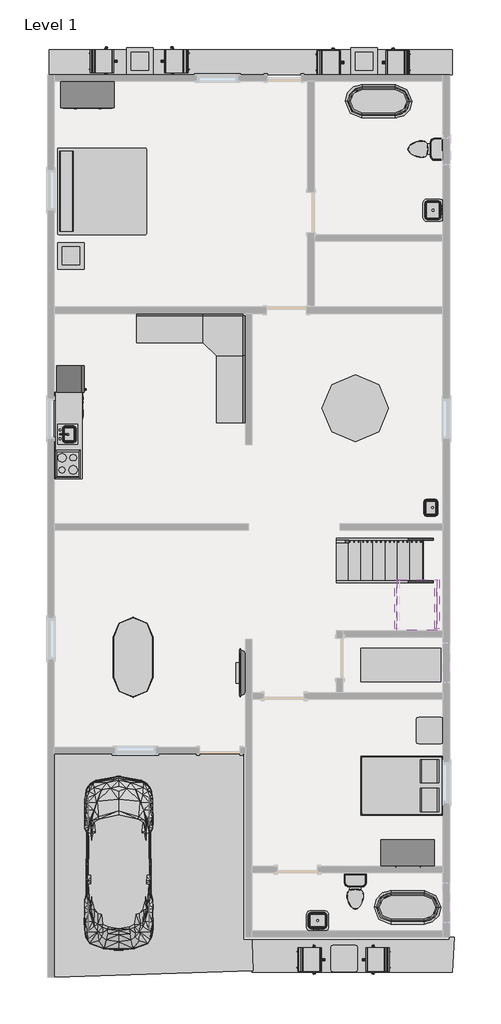
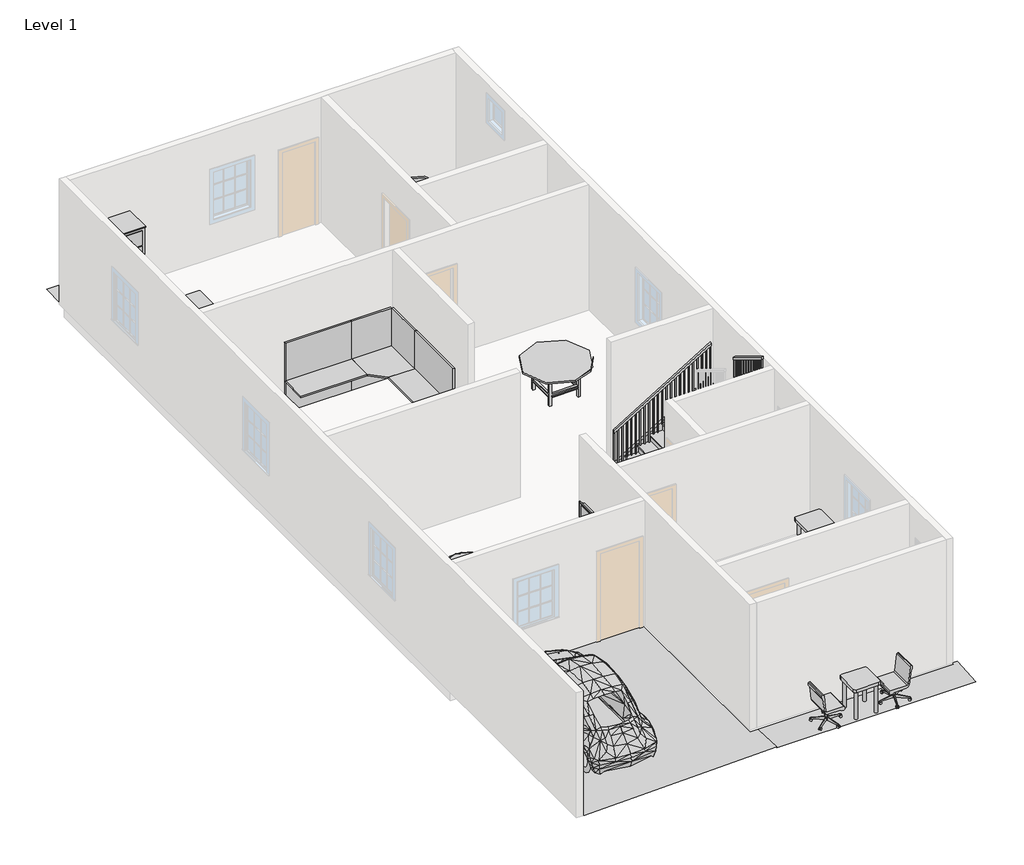
# One storey, part 2 of 2: 21 furniture elements, 8 flow terminals, 8 proxies, 4 members, 2 railings, 2 stair flights.
"""IFC4 building model written with IfcOpenShell, lengths in millimetres."""

from ifc_helpers import new_model, si_unit, frame, origin, place, context, project, spatial, polyline, outline, extrude, triangles, transform, mapped, element, save
from components import proxy_a6faaae8, proxy_45b28599, kitchenette_medium_kitchenette_medium_844211aa, rpc_beetle_rpc_beetle_3ce7ba48, proxy_c523a7b7, flow_terminal_871c2e40, flow_terminal_62a433f7, toilet_domestic_3d_toilet_domestic_3d_f7549cf7, toilet_domestic_3d_toilet_domestic_3d_183bbd19, flow_terminal_b374fae2, furniture_c8abb964, furniture_1fc5af50, chair_task_chair_task_b7f3823b, furniture_c6510c7c, furniture_9fa109b2, furniture_7a3aaa4f, furniture_b5c51a22, furniture_2c34a4f9, furniture_bbcc68ce, furniture_bcf351fa, furniture_a5b052b6, furniture_45e3acac, stair_flight_77e6af34, stair_flight_987ae6dc

model = new_model("IFC4")

# Units and contexts
model_context = context("Model", 3, world=origin())
ifc_project = project(units=[si_unit("LENGTHUNIT", "METRE", prefix="MILLI")], contexts=[model_context])

# Site, building, storey
site = spatial("IfcSite", under=ifc_project)
building = spatial("IfcBuilding", under=site)
storey = spatial("IfcBuildingStorey", under=building, Name="Level 1", Elevation=0.0)

# Proxies
placement = place(None, origin())
element("IfcBuildingElementProxy", 1, Name="Building Element Proxy", at=placement, inside=storey, context=model_context, shape_type="Tessellation", body=[
    triangles([(-7878.1871475, -7244.6450043, 0.0), (-7878.1871475, -8044.1648071, 0.0), (-3294.0675385, -8044.1648071, 0.0), (-3255.3873413, -7244.6450043, 0.0)], [[1, 2, 3], [3, 4, 1]], closed=False),
])
element("IfcBuildingElementProxy", 2, Name="Building Element Proxy", at=placement, inside=storey, context=model_context, shape_type="Tessellation", body=[
    triangles([(-12513.1071442, 13036.6751862, 0.0), (-12513.1071442, 12465.7553833, 0.0), (-3294.0675385, 13036.6751862, 0.0), (-3294.0675385, 12465.7553833, 0.0)], [[1, 2, 3], [4, 3, 2]], closed=False),
])
element("IfcBuildingElementProxy", 3, Name="Building Element Proxy", at=placement, inside=storey, context=model_context, shape_type="Tessellation", body=[
    triangles([(-12399.3873413, -3053.6450043, 0.0), (-8030.5871475, -3053.6450043, 0.0), (-7855.4362106, -8005.8386581, 0.0), (-12399.3873413, -8159.0450043, 0.0)], [[1, 4, 2], [3, 2, 4]], closed=False),
])
proxy_shape = proxy_a6faaae8(model_context)
element("IfcBuildingElementProxy", 4, Name="Cook Top-4 Unit2 : 22\" x 20\"", ObjectType="Cook Top-4 Unit2 : 22\" x 20\"", at=placement, inside=storey, context=model_context, shape_type="MappedRepresentation", body=[
    mapped(proxy_shape, transform((-12094.5873398, 3575.7549175, 0.0), x_axis=(0.0, 1.0000000000000002, 0.0), y_axis=(-1.0000000000000002, 0.0, 0.0), z_axis=(0.0, 0.0, 1.0))),
])
proxy_2_shape = proxy_45b28599(model_context)
element("IfcBuildingElementProxy", 5, Name="Dishwasher : 24\" x 24\" x 34\"", ObjectType="Dishwasher : 24\" x 24\" x 34\"", at=placement, inside=storey, context=model_context, shape_type="MappedRepresentation", body=[
    mapped(proxy_2_shape, transform((-11802.737775, 4526.937449, 0.0), x_axis=(0.0, 1.0000000000000002, 0.0), y_axis=(-1.0000000000000002, 0.0, 0.0), z_axis=(0.0, 0.0, 1.0))),
])
kitchenette_medium_kitchenette_medium_shape = kitchenette_medium_kitchenette_medium_844211aa(model_context)
element("IfcBuildingElementProxy", 6, Name="Kitchenette - Medium : Kitchenette - Medium", ObjectType="Kitchenette - Medium : Kitchenette - Medium", at=placement, inside=storey, context=model_context, shape_type="MappedRepresentation", body=[
    mapped(kitchenette_medium_kitchenette_medium_shape, transform((-12399.3873398, 3899.9172126, 0.0), x_axis=(0.0, 1.0000000000000002, 0.0), y_axis=(-1.0000000000000002, 0.0, 0.0), z_axis=(0.0, 0.0, 1.0))),
])
rpc_beetle_rpc_beetle_shape = rpc_beetle_rpc_beetle_3ce7ba48(model_context)
element("IfcBuildingElementProxy", 7, Name="RPC Beetle : RPC Beetle", ObjectType="RPC Beetle : RPC Beetle", at=placement, inside=storey, context=model_context, shape_type="MappedRepresentation", body=[
    mapped(rpc_beetle_rpc_beetle_shape, transform((-10926.1873398, -6787.4450825, 0.0), x_axis=(1.0, 0.0, 0.0), y_axis=(0.0, 1.0, 0.0), z_axis=(0.0, 0.0, 1.0))),
])
proxy_3_shape = proxy_c523a7b7(model_context)
element("IfcBuildingElementProxy", 8, Name="Refrigerator : 24\" x 25\" LH", ObjectType="Refrigerator : 24\" x 25\" LH", at=placement, inside=storey, context=model_context, shape_type="MappedRepresentation", body=[
    mapped(proxy_3_shape, transform((-12048.9383683, 5512.5049175, 0.0), x_axis=(0.0, 1.0000000000000002, 0.0), y_axis=(-1.0000000000000002, 0.0, 0.0), z_axis=(0.0, 0.0, 1.0))),
])

# Flow terminals
flow_terminal_shape = flow_terminal_871c2e40(model_context)
element("IfcFlowTerminal", 9, ObjectType="Sink Kitchen-Island : 18\" x 18\"", at=placement, inside=storey, context=model_context, shape_type="MappedRepresentation", body=[
    mapped(flow_terminal_shape, transform((-3753.0327409, 2588.1441581, 304.8), x_axis=(0.0, -1.0000000000000004, 0.0), y_axis=(1.0000000000000004, 0.0, 0.0), z_axis=(0.0, 0.0, 1.0))),
])
element("IfcFlowTerminal", 10, ObjectType="Sink Kitchen-Island : 18\" x 18\"", at=placement, inside=storey, context=model_context, shape_type="MappedRepresentation", body=[
    mapped(flow_terminal_shape, transform((-12092.2419387, 4233.165677, -14.4), x_axis=(0.0, 1.0000000000000002, 0.0), y_axis=(-1.0000000000000002, 0.0, 0.0), z_axis=(0.0, 0.0, 1.0))),
])
flow_terminal_2_shape = flow_terminal_62a433f7(model_context)
element("IfcFlowTerminal", 11, ObjectType="Sink Vanity-Square : 20\" x 18\"", at=placement, inside=storey, context=model_context, shape_type="MappedRepresentation", body=[
    mapped(flow_terminal_2_shape, transform((-6363.8980992, -6912.0996813, 304.8), x_axis=(-1.0, 0.0, 0.0), y_axis=(0.0, -1.0, 0.0), z_axis=(0.0, 0.0, 1.0))),
])
element("IfcFlowTerminal", 12, ObjectType="Sink Vanity-Square : 20\" x 18\"", at=placement, inside=storey, context=model_context, shape_type="MappedRepresentation", body=[
    mapped(flow_terminal_2_shape, transform((-3689.5327409, 9382.6441581, 304.8), x_axis=(0.0, -1.0000000000000002, 0.0), y_axis=(1.0000000000000002, 0.0, 0.0), z_axis=(0.0, 0.0, 1.0))),
])
toilet_domestic_3d_toilet_domestic_3d_shape = toilet_domestic_3d_toilet_domestic_3d_f7549cf7(model_context)
toilet_domestic_3d_toilet_domestic_3d_2_shape = toilet_domestic_3d_toilet_domestic_3d_183bbd19(model_context)
element("IfcFlowTerminal", 13, ObjectType="Toilet-Domestic-3D : Toilet-Domestic-3D", at=placement, inside=storey, context=model_context, shape_type="MappedRepresentation", body=[
    mapped(toilet_domestic_3d_toilet_domestic_3d_shape, transform((-5515.9873398, -6292.7490551, 0.0), x_axis=(1.0000000000000004, 0.0, 0.0), y_axis=(0.0, 1.0000000000000004, 0.0), z_axis=(0.0, 0.0, 1.0))),
    mapped(toilet_domestic_3d_toilet_domestic_3d_2_shape, transform((-5515.9873398, -6292.7490551, 0.0), x_axis=(1.0000000000000004, 0.0, 0.0), y_axis=(0.0, 1.0000000000000004, 0.0), z_axis=(0.0, 0.0, 1.0))),
])
element("IfcFlowTerminal", 14, ObjectType="Toilet-Domestic-3D : Toilet-Domestic-3D", at=placement, inside=storey, context=model_context, shape_type="MappedRepresentation", body=[
    mapped(toilet_domestic_3d_toilet_domestic_3d_shape, transform((-4004.0833671, 10763.9549175, 0.0), x_axis=(0.0, -1.0000000000000004, 0.0), y_axis=(1.0000000000000004, 0.0, 0.0), z_axis=(0.0, 0.0, 1.0))),
    mapped(toilet_domestic_3d_toilet_domestic_3d_2_shape, transform((-4004.0833671, 10763.9549175, 0.0), x_axis=(0.0, -1.0000000000000004, 0.0), y_axis=(1.0000000000000004, 0.0, 0.0), z_axis=(0.0, 0.0, 1.0))),
])
flow_terminal_3_shape = flow_terminal_b374fae2(model_context)
element("IfcFlowTerminal", 15, ObjectType="Tub-Free Standing-3D : 30\" x 60\"", at=placement, inside=storey, context=model_context, shape_type="MappedRepresentation", body=[
    mapped(flow_terminal_3_shape, transform((-4322.1873398, -6558.8450825, 0.0), x_axis=(0.0, -0.9999999999999998, 0.0), y_axis=(0.9999999999999998, 0.0, 0.0), z_axis=(0.0, 0.0, 1.0))),
])
element("IfcFlowTerminal", 16, ObjectType="Tub-Free Standing-3D : 30\" x 60\"", at=placement, inside=storey, context=model_context, shape_type="MappedRepresentation", body=[
    mapped(flow_terminal_3_shape, transform((-4982.5873398, 11856.1549175, 0.0), x_axis=(0.0, 1.0000000000000002, 0.0), y_axis=(-1.0000000000000002, 0.0, 0.0), z_axis=(0.0, 0.0, 1.0))),
])

# Furniture
furniture_shape = furniture_c8abb964(model_context)
element("IfcFurniture", 17, ObjectType="Bed-Box : Double 53\" x 74\"", at=placement, inside=storey, context=model_context, shape_type="MappedRepresentation", body=[
    mapped(furniture_shape, transform((-4214.7578316, -3438.3926234, 0.0), x_axis=(0.0, -1.0000000000000002, 0.0), y_axis=(1.0000000000000002, 0.0, 0.0), z_axis=(0.0, 0.0, 1.0))),
])
furniture_2_shape = furniture_1fc5af50(model_context)
element("IfcFurniture", 18, ObjectType="Bed-Standard : King 78\" x 80\"", at=placement, inside=storey, context=model_context, shape_type="MappedRepresentation", body=[
    mapped(furniture_2_shape, transform((-11352.7824218, 9527.266393, 0.0), x_axis=(0.0, 1.0000000000000002, 0.0), y_axis=(-1.0000000000000002, 0.0, 0.0), z_axis=(0.0, 0.0, 1.0))),
])
chair_task_chair_task_shape = chair_task_chair_task_b7f3823b(model_context)
element("IfcFurniture", 19, ObjectType="Chair-Task : Chair-Task", at=placement, inside=storey, context=model_context, shape_type="MappedRepresentation", body=[
    mapped(chair_task_chair_task_shape, transform((-4989.0414382, -7893.6359021, 0.0), x_axis=(0.0, 1.0000000000000009, 0.0), y_axis=(-1.0000000000000009, 0.0, 0.0), z_axis=(0.0, 0.0, 1.0))),
])
element("IfcFurniture", 20, ObjectType="Chair-Task : Chair-Task", at=placement, inside=storey, context=model_context, shape_type="MappedRepresentation", body=[
    mapped(chair_task_chair_task_shape, transform((-6576.3332414, -7611.6542628, 0.0), x_axis=(0.0, -1.0000000000000004, 0.0), y_axis=(1.0000000000000004, 0.0, 0.0), z_axis=(0.0, 0.0, 1.0))),
])
element("IfcFurniture", 21, ObjectType="Chair-Task : Chair-Task", at=placement, inside=storey, context=model_context, shape_type="MappedRepresentation", body=[
    mapped(chair_task_chair_task_shape, transform((-9586.4414382, 12629.5640979, 0.0), x_axis=(0.0, 1.0000000000000009, 0.0), y_axis=(-1.0000000000000009, 0.0, 0.0), z_axis=(0.0, 0.0, 1.0))),
])
element("IfcFurniture", 22, ObjectType="Chair-Task : Chair-Task", at=placement, inside=storey, context=model_context, shape_type="MappedRepresentation", body=[
    mapped(chair_task_chair_task_shape, transform((-11326.1332414, 12911.5457372, 0.0), x_axis=(0.0, -1.0000000000000009, 0.0), y_axis=(1.0000000000000009, 0.0, 0.0), z_axis=(0.0, 0.0, 1.0))),
])
element("IfcFurniture", 23, ObjectType="Chair-Task : Chair-Task", at=placement, inside=storey, context=model_context, shape_type="MappedRepresentation", body=[
    mapped(chair_task_chair_task_shape, transform((-6144.5332414, 12886.1457372, 0.0), x_axis=(0.0, -1.0000000000000007, 0.0), y_axis=(1.0000000000000007, 0.0, 0.0), z_axis=(0.0, 0.0, 1.0))),
])
element("IfcFurniture", 24, ObjectType="Chair-Task : Chair-Task", at=placement, inside=storey, context=model_context, shape_type="MappedRepresentation", body=[
    mapped(chair_task_chair_task_shape, transform((-4531.8414382, 12604.1640979, 0.0), x_axis=(0.0, 1.0000000000000007, 0.0), y_axis=(-1.0000000000000007, 0.0, 0.0), z_axis=(0.0, 0.0, 1.0))),
])
furniture_3_shape = furniture_c6510c7c(model_context)
element("IfcFurniture", 25, ObjectType="Counter Top w Sink Hole : 24\" Depth", at=placement, inside=storey, context=model_context, shape_type="MappedRepresentation", body=[
    mapped(furniture_3_shape, transform((-12399.3873398, 4433.3172126, -14.4), x_axis=(0.0, 1.0000000000000002, 0.0), y_axis=(-1.0000000000000002, 0.0, 0.0), z_axis=(0.0, 0.0, 1.0))),
])
furniture_4_shape = furniture_9fa109b2(model_context)
element("IfcFurniture", 26, ObjectType="Dresser : 48\" x 72\" x 24\"", at=placement, inside=storey, context=model_context, shape_type="MappedRepresentation", body=[
    mapped(furniture_4_shape, transform((-4052.99408, -4951.0821284, 0.0), x_axis=(1.0, 0.0, 0.0), y_axis=(0.0, 1.0, 0.0), z_axis=(0.0, 0.0, 1.0))),
])
element("IfcFurniture", 27, ObjectType="Dresser : 48\" x 72\" x 24\"", at=placement, inside=storey, context=model_context, shape_type="MappedRepresentation", body=[
    mapped(furniture_4_shape, transform((-11368.19408, 12371.7178716, 0.0), x_axis=(1.0, 0.0, 0.0), y_axis=(0.0, 1.0, 0.0), z_axis=(0.0, 0.0, 1.0))),
])
furniture_5_shape = furniture_7a3aaa4f(model_context)
element("IfcFurniture", 28, ObjectType="TV - Flat Screen : 42\"", at=placement, inside=storey, context=model_context, shape_type="MappedRepresentation", body=[
    mapped(furniture_5_shape, transform((-8089.1259634, -1203.3895966, 914.4), x_axis=(0.0, -1.0000000000000004, 0.0), y_axis=(1.0000000000000004, 0.0, 0.0), z_axis=(0.0, 0.0, 1.0))),
])
furniture_6_shape = furniture_b5c51a22(model_context)
element("IfcFurniture", 29, ObjectType="Table-Coffee : 24\" x 24\" x 24\"", at=placement, inside=storey, context=model_context, shape_type="MappedRepresentation", body=[
    mapped(furniture_6_shape, transform((-10461.8531065, 12675.3438397, 0.0), x_axis=(1.0, 0.0, 0.0), y_axis=(0.0, 1.0, 0.0), z_axis=(0.0, 0.0, 1.0))),
])
element("IfcFurniture", 30, ObjectType="Table-Coffee : 24\" x 24\" x 24\"", at=placement, inside=storey, context=model_context, shape_type="MappedRepresentation", body=[
    mapped(furniture_6_shape, transform((-5331.0531065, 12675.3438397, 0.0), x_axis=(1.0, 0.0, 0.0), y_axis=(0.0, 1.0, 0.0), z_axis=(0.0, 0.0, 1.0))),
])
element("IfcFurniture", 31, ObjectType="Table-Coffee : 24\" x 24\" x 24\"", at=placement, inside=storey, context=model_context, shape_type="MappedRepresentation", body=[
    mapped(furniture_6_shape, transform((-12036.6531065, 8230.3438397, 0.0), x_axis=(1.0, 0.0, 0.0), y_axis=(0.0, 1.0, 0.0), z_axis=(0.0, 0.0, 1.0))),
])
furniture_7_shape = furniture_2c34a4f9(model_context)
element("IfcFurniture", 32, ObjectType="Table-Dining Oval : 36\" x 72\"", at=placement, inside=storey, context=model_context, shape_type="MappedRepresentation", body=[
    mapped(furniture_7_shape, transform((-10954.0857004, -442.0254103, 0.0), x_axis=(0.0, 1.0000000000000002, 0.0), y_axis=(-1.0000000000000002, 0.0, 0.0), z_axis=(0.0, 0.0, 1.0))),
])
furniture_8_shape = furniture_bbcc68ce(model_context)
element("IfcFurniture", 33, ObjectType="Table-Dining Round w Chairs : 60\" Diameter", at=placement, inside=storey, context=model_context, shape_type="MappedRepresentation", body=[
    mapped(furniture_8_shape, transform((-5619.669307, 5030.6336061, 0.0), x_axis=(1.0, 0.0, 0.0), y_axis=(0.0, 1.0, 0.0), z_axis=(0.0, 0.0, 1.0))),
])
furniture_9_shape = furniture_bcf351fa(model_context)
element("IfcFurniture", 34, ObjectType="Table-End : 24\" x 24\"", at=placement, inside=storey, context=model_context, shape_type="MappedRepresentation", body=[
    mapped(furniture_9_shape, transform((-6078.5209701, -7879.6450825, 0.0), x_axis=(1.0, 0.0, 0.0), y_axis=(0.0, 1.0, 0.0), z_axis=(0.0, 0.0, 1.0))),
])
element("IfcFurniture", 35, ObjectType="Table-End : 24\" x 24\"", at=placement, inside=storey, context=model_context, shape_type="MappedRepresentation", body=[
    mapped(furniture_9_shape, transform((-4122.7209701, -2672.6450825, 0.0), x_axis=(1.0, 0.0, 0.0), y_axis=(0.0, 1.0, 0.0), z_axis=(0.0, 0.0, 1.0))),
])
furniture_10_shape = furniture_a5b052b6(model_context)
element("IfcFurniture", 36, ObjectType="Table-Rectangular : 72\" x 30\"", at=placement, inside=storey, context=model_context, shape_type="MappedRepresentation", body=[
    mapped(furniture_10_shape, transform((-4474.5873398, -1021.6450825, 0.0), x_axis=(1.0, 0.0, 0.0), y_axis=(0.0, 1.0, 0.0), z_axis=(0.0, 0.0, 1.0))),
])
furniture_11_shape = furniture_45e3acac(model_context)
element("IfcFurniture", 37, ObjectType="Work Station Cubicle : 96\" x 96\"", at=placement, inside=storey, context=model_context, shape_type="MappedRepresentation", body=[
    mapped(furniture_11_shape, transform((-7535.5643322, 6873.0231653, 0.0), x_axis=(0.0, -1.0000000000000004, 0.0), y_axis=(1.0000000000000004, 0.0, 0.0), z_axis=(0.0, 0.0, 1.0))),
])

# Members
element("IfcMember", 38, ObjectType="Stringer - 2\" Width", at=placement, inside=storey, context=model_context, shape_type="SweptSolid", body=[
    extrude(outline(polyline([(212.114512, -5947.7873398), (0.0, -5947.7873398), (0.0, -5709.701828), (1210.3724171, -3712.5873398), (1566.7811786, -3712.5873398), (212.114512, -5947.7873398)])), frame((0.0, 1823.1549175, 0.0), z_axis=(0.0, 1.0, 0.0), x_axis=(0.0, 0.0, 1.0)), (0.0, 0.0, 1.0), 50.8),
])
element("IfcMember", 39, ObjectType="Stringer - 2\" Width", at=placement, inside=storey, context=model_context, shape_type="SweptSolid", body=[
    extrude(outline(polyline([(212.114512, -5947.7873398), (0.0, -5947.7873398), (0.0, -5709.701828), (1210.3724171, -3712.5873398), (1566.7811786, -3712.5873398), (212.114512, -5947.7873398)])), frame((0.0, 857.9549175, 0.0), z_axis=(0.0, 1.0, 0.0), x_axis=(0.0, 0.0, 1.0)), (0.0, 0.0, 1.0), 50.8),
])
element("IfcMember", 40, ObjectType="Stringer - 2\" Width", at=placement, inside=storey, context=model_context, shape_type="SweptSolid", body=[
    extrude(outline(polyline([(923.5061342, 1736.114512), (923.5061342, 1379.7057504), (-194.0938658, 2057.0390838), (-194.0938658, 2413.4478453), (923.5061342, 1736.114512)])), frame((-3649.4448749, 0.0, 0.0), z_axis=(1.0, 0.0, 0.0), x_axis=(0.0, 1.0, 0.0)), (0.0, 0.0, 1.0), 50.8),
])
element("IfcMember", 41, ObjectType="Stringer - 2\" Width", at=placement, inside=storey, context=model_context, shape_type="SweptSolid", body=[
    extrude(outline(polyline([(923.5061342, 1736.114512), (923.5061342, 1379.7057504), (-194.0938658, 2057.0390838), (-194.0938658, 2413.4478453), (923.5061342, 1736.114512)])), frame((-4614.6448749, 0.0, 0.0), z_axis=(1.0, 0.0, 0.0), x_axis=(0.0, 1.0, 0.0)), (0.0, 0.0, 1.0), 50.8),
])

# Railings
element("IfcRailing", 42, ObjectType="Handrail - Rectangular", at=placement, inside=storey, context=model_context, shape_type="SweptSolid", body=[
    extrude(outline(polyline([(1083.7333333, -5947.7873398), (1024.3318731, -5947.7873398), (2378.9985397, -3712.5873398), (2438.4, -3712.5873398), (1083.7333333, -5947.7873398)])), frame((0.0, 1772.3549175, 0.0), z_axis=(0.0, 1.0, 0.0), x_axis=(0.0, 0.0, 1.0)), (0.0, 0.0, 1.0), 50.8),
    extrude(outline(polyline([(2311.6500549, -3823.7123398), (1354.6666667, -3823.7123398), (1354.6666667, -3804.6623398), (2323.1955094, -3804.6623398), (2311.6500549, -3823.7123398)])), frame((0.0, 1788.2299175, 0.0), z_axis=(0.0, 1.0, 0.0), x_axis=(0.0, 0.0, 1.0)), (0.0, 0.0, 1.0), 19.05),
    extrude(outline(polyline([(2250.0742973, -3925.3123398), (1354.6666667, -3925.3123398), (1354.6666667, -3906.2623398), (2261.6197519, -3906.2623398), (2250.0742973, -3925.3123398)])), frame((0.0, 1788.2299175, 0.0), z_axis=(0.0, 1.0, 0.0), x_axis=(0.0, 0.0, 1.0)), (0.0, 0.0, 1.0), 19.05),
    extrude(outline(polyline([(2188.4985397, -4026.9123398), (1185.3333333, -4026.9123398), (1185.3333333, -4007.8623398), (2200.0439943, -4007.8623398), (2188.4985397, -4026.9123398)])), frame((0.0, 1788.2299175, 0.0), z_axis=(0.0, 1.0, 0.0), x_axis=(0.0, 0.0, 1.0)), (0.0, 0.0, 1.0), 19.05),
    extrude(outline(polyline([(2126.9227822, -4128.5123398), (1185.3333333, -4128.5123398), (1185.3333333, -4109.4623398), (2138.4682367, -4109.4623398), (2126.9227822, -4128.5123398)])), frame((0.0, 1788.2299175, 0.0), z_axis=(0.0, 1.0, 0.0), x_axis=(0.0, 0.0, 1.0)), (0.0, 0.0, 1.0), 19.05),
    extrude(outline(polyline([(2065.3470246, -4230.1123398), (1185.3333333, -4230.1123398), (1185.3333333, -4211.0623398), (2076.8924791, -4211.0623398), (2065.3470246, -4230.1123398)])), frame((0.0, 1788.2299175, 0.0), z_axis=(0.0, 1.0, 0.0), x_axis=(0.0, 0.0, 1.0)), (0.0, 0.0, 1.0), 19.05),
    extrude(outline(polyline([(2003.771267, -4331.7123398), (1016.0, -4331.7123398), (1016.0, -4312.6623398), (2015.3167216, -4312.6623398), (2003.771267, -4331.7123398)])), frame((0.0, 1788.2299175, 0.0), z_axis=(0.0, 1.0, 0.0), x_axis=(0.0, 0.0, 1.0)), (0.0, 0.0, 1.0), 19.05),
    extrude(outline(polyline([(1942.1955094, -4433.3123398), (1016.0, -4433.3123398), (1016.0, -4414.2623398), (1953.740964, -4414.2623398), (1942.1955094, -4433.3123398)])), frame((0.0, 1788.2299175, 0.0), z_axis=(0.0, 1.0, 0.0), x_axis=(0.0, 0.0, 1.0)), (0.0, 0.0, 1.0), 19.05),
    extrude(outline(polyline([(1880.6197519, -4534.9123398), (1016.0, -4534.9123398), (1016.0, -4515.8623398), (1892.1652064, -4515.8623398), (1880.6197519, -4534.9123398)])), frame((0.0, 1788.2299175, 0.0), z_axis=(0.0, 1.0, 0.0), x_axis=(0.0, 0.0, 1.0)), (0.0, 0.0, 1.0), 19.05),
    extrude(outline(polyline([(1819.0439943, -4636.5123398), (846.6666667, -4636.5123398), (846.6666667, -4617.4623398), (1830.5894488, -4617.4623398), (1819.0439943, -4636.5123398)])), frame((0.0, 1788.2299175, 0.0), z_axis=(0.0, 1.0, 0.0), x_axis=(0.0, 0.0, 1.0)), (0.0, 0.0, 1.0), 19.05),
    extrude(outline(polyline([(1757.4682367, -4738.1123398), (846.6666667, -4738.1123398), (846.6666667, -4719.0623398), (1769.0136913, -4719.0623398), (1757.4682367, -4738.1123398)])), frame((0.0, 1788.2299175, 0.0), z_axis=(0.0, 1.0, 0.0), x_axis=(0.0, 0.0, 1.0)), (0.0, 0.0, 1.0), 19.05),
    extrude(outline(polyline([(1695.8924791, -4839.7123398), (846.6666667, -4839.7123398), (846.6666667, -4820.6623398), (1707.4379337, -4820.6623398), (1695.8924791, -4839.7123398)])), frame((0.0, 1788.2299175, 0.0), z_axis=(0.0, 1.0, 0.0), x_axis=(0.0, 0.0, 1.0)), (0.0, 0.0, 1.0), 19.05),
    extrude(outline(polyline([(1634.3167216, -4941.3123398), (677.3333333, -4941.3123398), (677.3333333, -4922.2623398), (1645.8621761, -4922.2623398), (1634.3167216, -4941.3123398)])), frame((0.0, 1788.2299175, 0.0), z_axis=(0.0, 1.0, 0.0), x_axis=(0.0, 0.0, 1.0)), (0.0, 0.0, 1.0), 19.05),
    extrude(outline(polyline([(1572.740964, -5042.9123398), (677.3333333, -5042.9123398), (677.3333333, -5023.8623398), (1584.2864185, -5023.8623398), (1572.740964, -5042.9123398)])), frame((0.0, 1788.2299175, 0.0), z_axis=(0.0, 1.0, 0.0), x_axis=(0.0, 0.0, 1.0)), (0.0, 0.0, 1.0), 19.05),
    extrude(outline(polyline([(1511.1652064, -5144.5123398), (508.0, -5144.5123398), (508.0, -5125.4623398), (1522.710661, -5125.4623398), (1511.1652064, -5144.5123398)])), frame((0.0, 1788.2299175, 0.0), z_axis=(0.0, 1.0, 0.0), x_axis=(0.0, 0.0, 1.0)), (0.0, 0.0, 1.0), 19.05),
    extrude(outline(polyline([(1449.5894488, -5246.1123398), (508.0, -5246.1123398), (508.0, -5227.0623398), (1461.1349034, -5227.0623398), (1449.5894488, -5246.1123398)])), frame((0.0, 1788.2299175, 0.0), z_axis=(0.0, 1.0, 0.0), x_axis=(0.0, 0.0, 1.0)), (0.0, 0.0, 1.0), 19.05),
    extrude(outline(polyline([(1388.0136913, -5347.7123398), (508.0, -5347.7123398), (508.0, -5328.6623398), (1399.5591458, -5328.6623398), (1388.0136913, -5347.7123398)])), frame((0.0, 1788.2299175, 0.0), z_axis=(0.0, 1.0, 0.0), x_axis=(0.0, 0.0, 1.0)), (0.0, 0.0, 1.0), 19.05),
    extrude(outline(polyline([(1326.4379337, -5449.3123398), (338.6666667, -5449.3123398), (338.6666667, -5430.2623398), (1337.9833882, -5430.2623398), (1326.4379337, -5449.3123398)])), frame((0.0, 1788.2299175, 0.0), z_axis=(0.0, 1.0, 0.0), x_axis=(0.0, 0.0, 1.0)), (0.0, 0.0, 1.0), 19.05),
    extrude(outline(polyline([(1264.8621761, -5550.9123398), (338.6666667, -5550.9123398), (338.6666667, -5531.8623398), (1276.4076307, -5531.8623398), (1264.8621761, -5550.9123398)])), frame((0.0, 1788.2299175, 0.0), z_axis=(0.0, 1.0, 0.0), x_axis=(0.0, 0.0, 1.0)), (0.0, 0.0, 1.0), 19.05),
    extrude(outline(polyline([(1203.2864185, -5652.5123398), (338.6666667, -5652.5123398), (338.6666667, -5633.4623398), (1214.8318731, -5633.4623398), (1203.2864185, -5652.5123398)])), frame((0.0, 1788.2299175, 0.0), z_axis=(0.0, 1.0, 0.0), x_axis=(0.0, 0.0, 1.0)), (0.0, 0.0, 1.0), 19.05),
    extrude(outline(polyline([(1141.710661, -5754.1123398), (169.3333333, -5754.1123398), (169.3333333, -5735.0623398), (1153.2561155, -5735.0623398), (1141.710661, -5754.1123398)])), frame((0.0, 1788.2299175, 0.0), z_axis=(0.0, 1.0, 0.0), x_axis=(0.0, 0.0, 1.0)), (0.0, 0.0, 1.0), 19.05),
    extrude(outline(polyline([(1080.1349034, -5855.7123398), (169.3333333, -5855.7123398), (169.3333333, -5836.6623398), (1091.6803579, -5836.6623398), (1080.1349034, -5855.7123398)])), frame((0.0, 1788.2299175, 0.0), z_axis=(0.0, 1.0, 0.0), x_axis=(0.0, 0.0, 1.0)), (0.0, 0.0, 1.0), 19.05),
    extrude(outline(polyline([(2367.4530852, -3731.6373398), (1354.6666667, -3731.6373398), (1354.6666667, -3712.5873398), (2378.9985397, -3712.5873398), (2367.4530852, -3731.6373398)])), frame((0.0, 1788.2299175, 0.0), z_axis=(0.0, 1.0, 0.0), x_axis=(0.0, 0.0, 1.0)), (0.0, 0.0, 1.0), 19.05),
    extrude(outline(polyline([(1024.3318731, -5947.7873398), (169.3333333, -5947.7873398), (169.3333333, -5928.7373398), (1035.8773276, -5928.7373398), (1024.3318731, -5947.7873398)])), frame((0.0, 1788.2299175, 0.0), z_axis=(0.0, 1.0, 0.0), x_axis=(0.0, 0.0, 1.0)), (0.0, 0.0, 1.0), 19.05),
])
element("IfcRailing", 43, ObjectType="Handrail - Rectangular", at=placement, inside=storey, context=model_context, shape_type="SweptSolid", body=[
    extrude(outline(polyline([(923.5061342, 2607.7333333), (923.5061342, 2548.3318731), (-194.0938658, 3225.6652064), (-194.0938658, 3285.0666667), (923.5061342, 2607.7333333)])), frame((-3700.2448749, 0.0, 0.0), z_axis=(1.0, 0.0, 0.0), x_axis=(0.0, 1.0, 0.0)), (0.0, 0.0, 1.0), 50.8),
    extrude(outline(polyline([(812.3811342, 2615.6803579), (831.4311342, 2604.1349034), (831.4311342, 1693.3333333), (812.3811342, 1693.3333333), (812.3811342, 2615.6803579)])), frame((-3684.3698749, 0.0, 0.0), z_axis=(1.0, 0.0, 0.0), x_axis=(0.0, 1.0, 0.0)), (0.0, 0.0, 1.0), 19.05),
    extrude(outline(polyline([(710.7811342, 2677.2561155), (729.8311342, 2665.710661), (729.8311342, 1693.3333333), (710.7811342, 1693.3333333), (710.7811342, 2677.2561155)])), frame((-3684.3698749, 0.0, 0.0), z_axis=(1.0, 0.0, 0.0), x_axis=(0.0, 1.0, 0.0)), (0.0, 0.0, 1.0), 19.05),
    extrude(outline(polyline([(609.1811342, 2738.8318731), (628.2311342, 2727.2864185), (628.2311342, 1862.6666667), (609.1811342, 1862.6666667), (609.1811342, 2738.8318731)])), frame((-3684.3698749, 0.0, 0.0), z_axis=(1.0, 0.0, 0.0), x_axis=(0.0, 1.0, 0.0)), (0.0, 0.0, 1.0), 19.05),
    extrude(outline(polyline([(507.5811342, 2800.4076307), (526.6311342, 2788.8621761), (526.6311342, 1862.6666667), (507.5811342, 1862.6666667), (507.5811342, 2800.4076307)])), frame((-3684.3698749, 0.0, 0.0), z_axis=(1.0, 0.0, 0.0), x_axis=(0.0, 1.0, 0.0)), (0.0, 0.0, 1.0), 19.05),
    extrude(outline(polyline([(405.9811342, 2861.9833882), (425.0311342, 2850.4379337), (425.0311342, 1862.6666667), (405.9811342, 1862.6666667), (405.9811342, 2861.9833882)])), frame((-3684.3698749, 0.0, 0.0), z_axis=(1.0, 0.0, 0.0), x_axis=(0.0, 1.0, 0.0)), (0.0, 0.0, 1.0), 19.05),
    extrude(outline(polyline([(304.3811342, 2923.5591458), (323.4311342, 2912.0136913), (323.4311342, 2032.0), (304.3811342, 2032.0), (304.3811342, 2923.5591458)])), frame((-3684.3698749, 0.0, 0.0), z_axis=(1.0, 0.0, 0.0), x_axis=(0.0, 1.0, 0.0)), (0.0, 0.0, 1.0), 19.05),
    extrude(outline(polyline([(202.7811342, 2985.1349034), (221.8311342, 2973.5894488), (221.8311342, 2032.0), (202.7811342, 2032.0), (202.7811342, 2985.1349034)])), frame((-3684.3698749, 0.0, 0.0), z_axis=(1.0, 0.0, 0.0), x_axis=(0.0, 1.0, 0.0)), (0.0, 0.0, 1.0), 19.05),
    extrude(outline(polyline([(101.1811342, 3046.710661), (120.2311342, 3035.1652064), (120.2311342, 2032.0), (101.1811342, 2032.0), (101.1811342, 3046.710661)])), frame((-3684.3698749, 0.0, 0.0), z_axis=(1.0, 0.0, 0.0), x_axis=(0.0, 1.0, 0.0)), (0.0, 0.0, 1.0), 19.05),
    extrude(outline(polyline([(-0.4188658, 3108.2864185), (18.6311342, 3096.740964), (18.6311342, 2201.3333333), (-0.4188658, 2201.3333333), (-0.4188658, 3108.2864185)])), frame((-3684.3698749, 0.0, 0.0), z_axis=(1.0, 0.0, 0.0), x_axis=(0.0, 1.0, 0.0)), (0.0, 0.0, 1.0), 19.05),
    extrude(outline(polyline([(-102.0188658, 3169.8621761), (-82.9688658, 3158.3167216), (-82.9688658, 2201.3333333), (-102.0188658, 2201.3333333), (-102.0188658, 3169.8621761)])), frame((-3684.3698749, 0.0, 0.0), z_axis=(1.0, 0.0, 0.0), x_axis=(0.0, 1.0, 0.0)), (0.0, 0.0, 1.0), 19.05),
    extrude(outline(polyline([(904.4561342, 2559.8773276), (923.5061342, 2548.3318731), (923.5061342, 1693.3333333), (904.4561342, 1693.3333333), (904.4561342, 2559.8773276)])), frame((-3684.3698749, 0.0, 0.0), z_axis=(1.0, 0.0, 0.0), x_axis=(0.0, 1.0, 0.0)), (0.0, 0.0, 1.0), 19.05),
    extrude(outline(polyline([(-194.0938658, 3225.6652064), (-175.0438658, 3214.1197519), (-175.0438658, 2201.3333333), (-194.0938658, 2201.3333333), (-194.0938658, 3225.6652064)])), frame((-3684.3698749, 0.0, 0.0), z_axis=(1.0, 0.0, 0.0), x_axis=(0.0, 1.0, 0.0)), (0.0, 0.0, 1.0), 19.05),
])

# Stair flights
stair_flight_shape = stair_flight_77e6af34(model_context)
element("IfcStairFlight", 44, ObjectType="2\" Tread 1\" Nosing 1/4\" Riser", at=placement, inside=storey, context=model_context, shape_type="MappedRepresentation", body=[
    mapped(stair_flight_shape, transform((0.0, 0.0, 0.0), x_axis=(1.0, 0.0, 0.0), y_axis=(0.0, 1.0, 0.0), z_axis=(0.0, 0.0, 1.0))),
])
stair_flight_2_shape = stair_flight_987ae6dc(model_context)
element("IfcStairFlight", 45, ObjectType="2\" Tread 1\" Nosing 1/4\" Riser", at=placement, inside=storey, context=model_context, shape_type="MappedRepresentation", body=[
    mapped(stair_flight_2_shape, transform((0.0, 0.0, 0.0), x_axis=(1.0, 0.0, 0.0), y_axis=(0.0, 1.0, 0.0), z_axis=(0.0, 0.0, 1.0))),
])

save(model, "model.ifc")

# Revit data of these elements
# Type "Cook Top-4 Unit2 : 22\" x 20\""
#   Depth = 1' - 8"
#   Width = 1' - 10"
#   Burner Material = Steel, Chrome Plated
#   Cooktop Material = Steel, Polished
#   Default Elevation = 0
#   Assembly Code = ""
# Type "Dishwasher : 24\" x 24\" x 34\""
#   Label = "DW"
#   Assembly Code = "E1090400"
#   Depth = 2' - 0"
#   Height = 2' - 10"
#   Width = 2' - 0"
#   Dishwasher Material = Steel, Paint Finish, Ivory, Glossy
#   Panel Face Material = Plastic, Opaque Black
#   Default Elevation = 0
# Type "Kitchenette - Medium : Kitchenette - Medium"
#   Assembly Code = "E1090400"
#   Counter Length = 6' - 6"
#   Cabinet Width = 4' - 6"
#   Cabinet Height = 2' - 10 1/2"
#   Cabinet Depth = 2' - 0"
#   Toe Depth = 0' - 3"
#   Toe Height = 0' - 3 1/2"
#   Cabinet Material = Cabinets
#   Door/Drawer Material = Cabinets
#   Handle Material = Cabinets - Handles
#   Default Elevation = 0
# Type "RPC Beetle : RPC Beetle"
#   built-in parameter 1005195 = "RPC-16-0U6E-L4EG-ENH1-J3KF-SVEL-0TX4-C0"
#   Height = 0
# Type "Refrigerator : 24\" x 25\" LH"
#   Label = "REF."
#   Assembly Code = "E1090400"
#   Depth = 2' - 0 3/4"
#   Handle = 0' - 1 1/2"
#   Height = 5' - 3 1/2"
#   Rear Clearance = 0' - 2"
#   Top Door Height = 1' - 8"
#   Width = 1' - 11 1/2"
#   Material = Steel, Paint Finish, Ivory, Glossy
#   Default Elevation = 0
# Type "Sink Kitchen-Island : 18\" x 18\""
#   Assembly Code = "D2010410"
#   Counter Height = 3' - 0"
#   Depth = 1' - 6"
#   Width = 1' - 6"
#   Faucet Material = Steel, Polished
#   Sink Material = Steel, Polished
#   Default Elevation = 0
# Type "Sink Vanity-Square : 20\" x 18\""
#   Assembly Code = "D2010400"
#   Counter Height = 2' - 7"
#   Depth = 1' - 6"
#   Width = 1' - 8"
#   Basin Material = Porcelain, Linen
#   Faucet Material = Steel, Polished
#   Default Elevation = 0
# Type "Toilet-Domestic-3D : Toilet-Domestic-3D"
#   Assembly Code = "D2010110"
#   Toilet - Bowl/Basin Material = Porcelain, Linen
#   Toilet - Seat Material = Laminate, Linen, Matte
#   Default Elevation = 0
# Type "Tub-Free Standing-3D : 30\" x 60\""
#   Assembly Code = "D2010110"
#   Height = 1' - 6"
#   Length = 5' - 0"
#   Width = 2' - 6"
#   Tub Material = Porcelain, Ivory
#   Default Elevation = 0
# Type "Bed-Box : Double 53\" x 74\""
#   Assembly Code = "E2020200"
#   Length = 6' - 2"
#   Width = 4' - 5"
#   Frame Material = Birch
#   Mattress Material = Linen, White
#   Default Elevation = 0
# Type "Bed-Standard : King 78\" x 80\""
#   Assembly Code = "E2020200"
#   Length = 6' - 8"
#   Width = 6' - 6"
#   Leg Material = Steel, Chrome Plated
#   Mattress Material = Linen, White
#   Default Elevation = 0
# Type "Chair-Task : Chair-Task"
#   Assembly Code = "E2020200"
#   Base Material = Plastic, Opaque Black
#   Caster Material = Plastic, Opaque Black
#   Seat/Back Material = Textile - Slate Blue
#   Default Elevation = 0
# Type "Counter Top w Sink Hole : 24\" Depth"
#   Assembly Code = "C1030400"
#   Counter Thickness = 0' - 1 1/2"
#   Depth = 2' - 1"
#   Height = 3' - 0"
#   Length [instance default] = 8' - 0"
#   Sink Location [instance default] = 2' - 0"
#   Sink Location To Wall [instance default] = 0' - 6"
#   Sink Opening Depth [instance default] = 1' - 3"
#   Sink Opening Width [instance default] = 2' - 3"
#   Counter Top Material = none
#   Default Elevation = 0
# Type "Dresser : 48\" x 72\" x 24\""
#   Assembly Code = "E2020200"
#   Depth = 2' - 0"
#   Height = 6' - 0"
#   Width = 4' - 0"
#   Dresser Material = Laminate - Ivory, Glossy
#   Drawer Material = Laminate, Ivory, Matte
#   Knob Material = Cherry
#   Default Elevation = 0
# Type "TV - Flat Screen : 42\""
#   SinAng = 0' - 0.0193"
#   L = 3' - 0.71517"
#   H = 1' - 8.65418"
#   Thickness = 0' - 4.33071"
#   Diagonal = 3' - 6.12598"
#   CosAng = 0' - 0.03431"
#   Stand [instance default] = yes
#   Default Elevation = 0
# Type "Table-Coffee : 24\" x 24\" x 24\""
#   Assembly Code = "E2020200"
#   Height = 2' - 0"
#   Length = 2' - 0"
#   Width = 2' - 0"
#   Top Material = none
#   Frame Material = none
#   Default Elevation = 0
# Type "Table-Dining Oval : 36\" x 72\""
#   Assembly Code = "E2020200"
#   Length = 6' - 0"
#   Width = 3' - 0"
#   Base Material = Steel, Chrome Plated
#   Top Material = Glass - Clear, Grey
#   Default Elevation = 0
#   Description = (empty or 0)
# Type "Table-Dining Round w Chairs : 60\" Diameter"
#   Assembly Code = "E2020200"
#   Radius = 2' - 6"
#   Diameter = 5' - 0"
#   Height = 2' - 6"
#   Chairs = 6
#   Base Material = Pine
#   Top Material = Laminate, Linen, Matte
#   Default Elevation = 0
# Type "Table-End : 24\" x 24\""
#   Assembly Code = "E2020200"
#   Height = 2' - 6"
#   Length = 2' - 0"
#   Width = 2' - 0"
#   Base Material = Birch
#   Top Material = Laminate, Ivory, Matte
#   Default Elevation = 0
# Type "Table-Rectangular : 72\" x 30\""
#   Assembly Code = "E2020200"
#   Height = 2' - 6"
#   Length = 6' - 0"
#   Width = 2' - 6"
#   Base Material = Birch
#   Top Material = Birch
#   Default Elevation = 0
# Type "Work Station Cubicle : 96\" x 96\""
#   Assembly Code = "E2020"
#   Desktop Height = 2' - 6"
#   Desktop1 Width = 2' - 0"
#   Desktop2 Width = 2' - 0"
#   Panel Height = 5' - 6"
#   Panel1 Length = 5' - 0"
#   Panel2 Length = 5' - 0"
#   Cube Panel Material = Textile - Light Gray
#   Work Top Material = Laminate, Ivory, Matte
#   Default Elevation = 0
# Type "Handrail - Rectangular"
#   Assembly Code = "C2010400"
#   built-in parameter 1008612 = 0.0416667 (stored number, unit not read)
#   built-in parameter 1008611 = 0.0416667 (stored number, unit not read)
#   built-in parameter 1008609 = 0.333333 (stored number, unit not read)
#   built-in parameter 1008604 = 0.166667 (stored number, unit not read)
#   built-in parameter 1008603 = 0.166667 (stored number, unit not read)
#   Railing Height = 3' - 0"
#   built-in parameter 1008630 = 2
#   built-in parameter 1008610 = 2
#   built-in parameter 1008618 = Baluster - Square : 3/4"
# Elements 1, 2, 3 (IfcBuildingElementProxy)
#   Material = none
#   Phase Created = New Construction
# Element 4 (IfcBuildingElementProxy, "Cook Top-4 Unit2 : 22\" x 20\"")
#   Phase Created = New Construction
#   Materials on its faces: "Steel, Chrome Plated", "Steel, Polished"
# Element 5 (IfcBuildingElementProxy, "Dishwasher : 24\" x 24\" x 34\"")
#   Phase Created = New Construction
#   Materials on its faces: "Steel, Paint Finish, Ivory, Glossy", "Plastic, Opaque Black"
# Element 6 (IfcBuildingElementProxy, "Kitchenette - Medium : Kitchenette - Medium")
#   Phase Created = New Construction
#   Materials on its faces: "Cabinets", "Cabinets - Handles"
# Element 7 (IfcBuildingElementProxy, "RPC Beetle : RPC Beetle")
#   Phase Created = New Construction
# Element 8 (IfcBuildingElementProxy, "Refrigerator : 24\" x 25\" LH")
#   Phase Created = New Construction
#   Materials on its faces: "Steel, Paint Finish, Ivory, Glossy", "Steel, Chrome Plated"
# Element 9 (IfcFlowTerminal, "Sink Kitchen-Island : 18\" x 18\"")
#   Mark = "4"
#   Phase Created = New Construction
#   Materials on its faces: "Steel, Polished"
# Element 10 (IfcFlowTerminal, "Sink Kitchen-Island : 18\" x 18\"")
#   Mark = "5"
#   Phase Created = New Construction
#   Materials on its faces: "Steel, Polished"
# Element 11 (IfcFlowTerminal, "Sink Vanity-Square : 20\" x 18\"")
#   Mark = "3"
#   Phase Created = New Construction
#   Materials on its faces: "Porcelain, Linen", "Steel, Polished"
# Element 12 (IfcFlowTerminal, "Sink Vanity-Square : 20\" x 18\"")
#   Mark = "8"
#   Phase Created = New Construction
#   Materials on its faces: "Porcelain, Linen", "Steel, Polished"
# Element 13 (IfcFlowTerminal, "Toilet-Domestic-3D : Toilet-Domestic-3D")
#   Mark = "1"
#   Phase Created = New Construction
#   Materials on its faces: "Porcelain, Linen", "Laminate, Linen, Matte"
# Element 14 (IfcFlowTerminal, "Toilet-Domestic-3D : Toilet-Domestic-3D")
#   Mark = "7"
#   Phase Created = New Construction
#   Materials on its faces: "Porcelain, Linen", "Laminate, Linen, Matte"
# Element 15 (IfcFlowTerminal, "Tub-Free Standing-3D : 30\" x 60\"")
#   Mark = "2"
#   Phase Created = New Construction
#   Materials on its faces: "Porcelain, Ivory"
# Element 16 (IfcFlowTerminal, "Tub-Free Standing-3D : 30\" x 60\"")
#   Mark = "6"
#   Phase Created = New Construction
#   Materials on its faces: "Porcelain, Ivory"
# Element 17 (IfcFurniture, "Bed-Box : Double 53\" x 74\"")
#   Phase Created = New Construction
#   Materials on its faces: "Birch", "Linen, White"
# Element 18 (IfcFurniture, "Bed-Standard : King 78\" x 80\"")
#   Phase Created = New Construction
#   Materials on its faces: "Linen, White", "Steel, Chrome Plated"
# Elements 19, 20, 21, 22, 23, 24 (IfcFurniture, "Chair-Task : Chair-Task")
#   Phase Created = New Construction
#   Materials on its faces: "Plastic, Opaque Black", "Textile - Slate Blue"
# Element 25 (IfcFurniture, "Counter Top w Sink Hole : 24\" Depth")
#   Sink Opening Depth = 1' - 2"
#   Sink Location To Wall = 0' - 6"
#   Length = 6' - 6"
#   Sink Location = 3' - 4"
#   Sink Opening Width = 1' - 4"
#   Phase Created = New Construction
#   Materials on its faces: "Counter Top"
# Elements 26, 27 (IfcFurniture, "Dresser : 48\" x 72\" x 24\"")
#   Phase Created = New Construction
#   Materials on its faces: "Laminate, Ivory, Matte", "Cherry", "Laminate - Ivory, Glossy"
# Element 28 (IfcFurniture, "TV - Flat Screen : 42\"")
#   Stand = yes
#   Phase Created = New Construction
#   Materials on its faces: "TV - Black", "TV - Glass", "TV - Screen"
# Elements 29, 30, 31 (IfcFurniture, "Table-Coffee : 24\" x 24\" x 24\"")
#   Phase Created = New Construction
#   Materials on its faces: "Glass - Clear, Grey"
# Element 32 (IfcFurniture, "Table-Dining Oval : 36\" x 72\"")
#   Phase Created = New Construction
#   Materials on its faces: "Steel, Chrome Plated", "Glass - Clear, Grey"
# Element 33 (IfcFurniture, "Table-Dining Round w Chairs : 60\" Diameter")
#   Phase Created = New Construction
#   Materials on its faces: "Pine", "Laminate, Linen, Matte"
# Elements 34, 35 (IfcFurniture, "Table-End : 24\" x 24\"")
#   Phase Created = New Construction
#   Materials on its faces: "Laminate, Ivory, Matte", "Birch"
# Element 36 (IfcFurniture, "Table-Rectangular : 72\" x 30\"")
#   Phase Created = New Construction
#   Materials on its faces: "Birch"
# Element 37 (IfcFurniture, "Work Station Cubicle : 96\" x 96\"")
#   Phase Created = New Construction
#   Materials on its faces: "Textile - Light Gray", "Laminate, Ivory, Matte"
# Elements 38, 39, 40, 41 (IfcMember, "Stringer - 2\" Width")
#   Phase Created = New Construction
# Elements 42, 43 (IfcRailing, "Handrail - Rectangular")
#   Phase Created = New Construction
# Elements 44, 45 (IfcStairFlight, "2\" Tread 1\" Nosing 1/4\" Riser")
#   Phase Created = New Construction
# Materials
#   "Steel, Chrome Plated": class "Metal", colour RGB 17 17 17, transparency 0, Description = "Chromiuim plated steel", Cost = 0
#   "Steel, Polished": class "Metal", colour RGB 57 57 57, transparency 0, Description = "Polished steel", Cost = 0
#   "Steel, Paint Finish, Ivory, Glossy": class "Metal", colour RGB 247 247 239, transparency 0, Description = "Steel, paint finish, ivory, glossy", Cost = 0
#   "Plastic, Opaque Black": class "Plastic", colour RGB 0 0 0, transparency 0.7, Description = "Plastic, generic, opaque black", Cost = 0
#   "Cabinets": colour RGB 249 249 249, transparency 0
#   "Cabinets - Handles": class "Metal", colour RGB 57 57 57, transparency 0
#   "Porcelain, Linen": class "Ceramic", colour RGB 249 239 230, transparency 0, Description = "Porcelain, linen", Cost = 0
#   "Laminate, Linen, Matte": class "Plastic", colour RGB 249 239 230, transparency 0, Description = "Plastic Laminate - Linen, Matte", Cost = 0
#   "Porcelain, Ivory": class "Ceramic", colour RGB 247 247 239, transparency 0, Description = "Porcelain, ivory", Cost = 0
#   "Birch": class "Wood", colour RGB 224 178 126, transparency 0, Description = "Betula Alleghaniensis", Cost = 0
#   "Linen, White": class "Textile", colour RGB 247 247 239, transparency 0, Description = "Linen, white", Cost = 0
#   "Textile - Slate Blue": class "Fabric", colour RGB 98 102 118, transparency 0
#   "Laminate - Ivory, Glossy": colour RGB 247 247 239, transparency 0
#   "Laminate, Ivory, Matte": class "Plastic", colour RGB 247 247 239, transparency 0, Description = "Plastic Laminate - Ivory, Matte", Cost = 0
#   "Cherry": class "Wood", colour RGB 226 177 128, transparency 0, Description = "Prunus Serotina", Cost = 0
#   "Glass - Clear, Grey": class "Glass", colour RGB 252 255 255, transparency 0.64
#   "Pine": class "Wood", colour RGB 223 192 134, transparency 0, Description = "Pinus Echinata", Cost = 0
#   "Textile - Light Gray": class "Fabric", colour RGB 204 204 204, transparency 0
#   "Counter Top": class "Wood", colour RGB 226 177 128, transparency 0
#   "TV - Black": colour RGB 49 49 49, transparency 0
#   "TV - Glass": colour RGB 157 157 157, transparency 0.9
#   "TV - Screen": colour RGB 0 0 0, transparency 0
